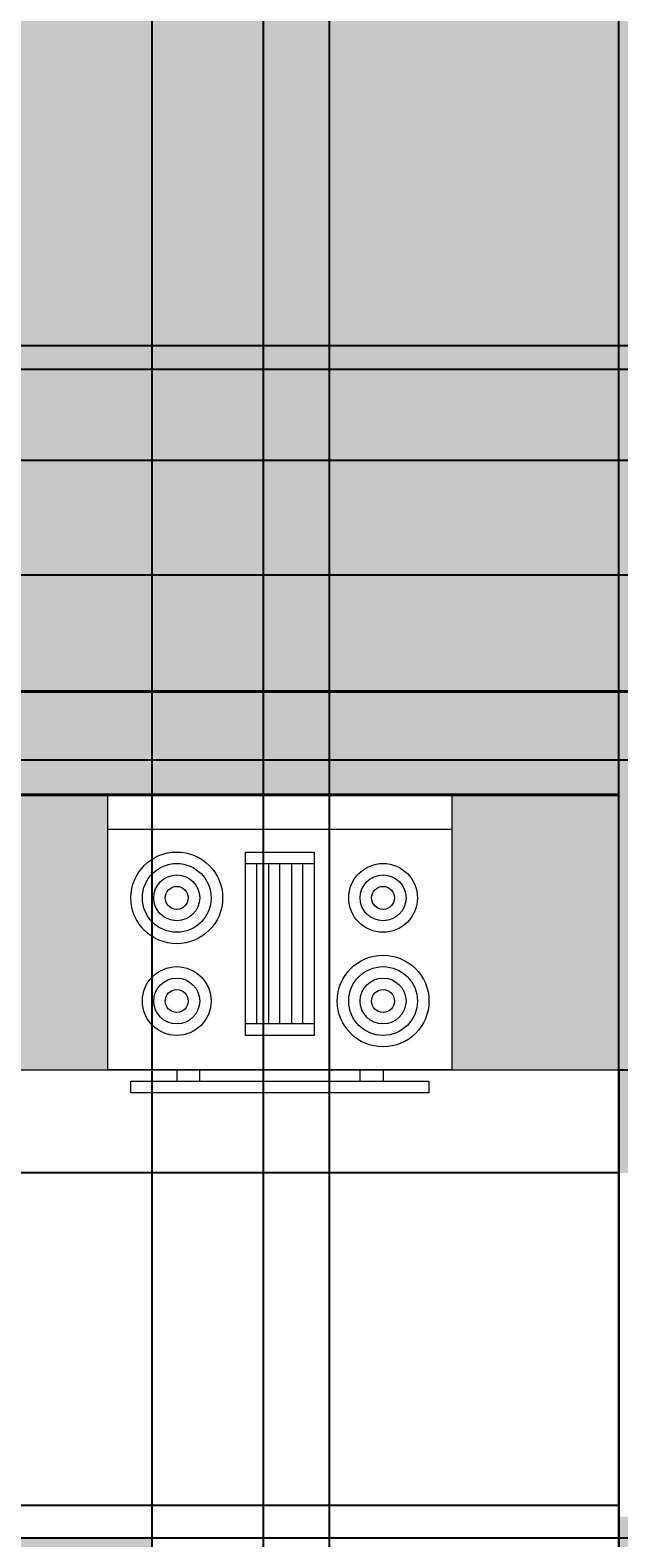
# Model space of a CAD drawing. Units: inches. Extents: x 818 to 1898, y 976 to 2364.
# Tile 87 of 96: x 1539 to 1591, y 1979 to 2111. Entities that reach past the tile are written whole.
import ezdxf

# ---------------------------------------------------------------- set-up
doc = ezdxf.new("R2010")
doc.units = ezdxf.units.IN
doc.header["$LTSCALE"] = 5
doc.header["$MEASUREMENT"] = 0
for name, color, linetype, lineweight in [('A-ANNO-DIMS', 2, 'Continuous', 18), ('A-EQPM', 8, 'Continuous', 18), ('A-FLOR-CASE', 8, 'Continuous', 18), ('A-FURN-PATT', 8, 'Continuous', 9), ('A-WALL', 7, 'Continuous', 40)]:
    doc.layers.add(name, color=color, linetype=linetype, lineweight=lineweight)
doc.layers.add('A-WALL-PATT', color=251, linetype='Continuous', lineweight=13, true_color=0x636466)
doc.layers.add('L-PLNT-PATT', color=114, linetype='Continuous', lineweight=9, true_color=0x139b48)
doc.styles.get("Standard").update_dxf_attribs({"font": 'arial.ttf'})
doc.dimstyles.get("Standard").update_dxf_attribs({"dimtxt": 0.18, "dimasz": 0.18, "dimexe": 0.18, "dimexo": 0.0625, "dimgap": 0.09, "dimtad": 0, "dimtih": 1, "dimtoh": 1, "dimdec": 4, "dimzin": 0, "dimdsep": 46, "dimtxsty": 'Standard', "dimcen": 0.09, "dimadec": 0, "dimazin": 0, "dimtfac": 1, "dimtdec": 4, "dimtofl": 0, "dimtmove": 0, "dimatfit": 3, "dimfxl": 1, "dimtolj": 1, "dimtzin": 0, "dimarcsym": 0})

# ---------------------------------------------------------------- blocks, each defined once
blk = doc.blocks.new('Range-Oven - 30 in top')
for p, q in [((0, -3), (30, -3)), ((12, -6), (18, -6)), ((13, -20), (13, -6)), ((14, -6), (14, -20)), ((15, -20), (15, -6)), ((16, -6), (16, -20)), ((17, -20), (17, -6)), ((18, -20), (12, -20)), ((6, -24), (6, -25)), ((8, -25), (8, -24)), ((22, -25), (22, -24)), ((24, -24), (24, -25))]:
    blk.add_line(p, q)
for points in [[(0, -24), (0, 0), (30, 0), (30, -24)], [(12, -21), (12, -5), (18, -5), (18, -21)], [(2, -26), (2, -25), (28, -25), (28, -26)]]:
    blk.add_lwpolyline(points, close=True)
for centre, radius in [((6, -9), 4), ((6, -9), 3), ((24, -9), 3), ((6, -9), 2), ((24, -9), 2), ((6, -9), 1), ((24, -9), 1), ((24, -18), 4), ((6, -18), 3), ((24, -18), 3), ((6, -18), 2), ((6, -18), 1), ((24, -18), 2), ((24, -18), 1)]:
    blk.add_circle(centre, radius)
blk = doc.blocks.new('*D73')
at = {"layer": 'A-ANNO-DIMS', "color": 0, "lineweight": -2, "ltscale": 5, "transparency": 16777216}
for p, q in [((1590.66, 2011.08), (818.03, 2011.08)), ((818.21, 2010.9), (818.21, 1996.76)), ((818.21, 1982.26), (818.21, 1996.4)), ((1590.66, 1982.08), (818.03, 1982.08))]:
    blk.add_line(p, q, dxfattribs=at)
at = {"layer": 'A-ANNO-DIMS', "color": 0, "ltscale": 5, "transparency": 16777216}
for points in [[(818.18, 2010.9), (818.24, 2010.9), (818.21, 2011.08)], [(818.18, 1982.26), (818.24, 1982.26), (818.21, 1982.08)]]:
    blk.add_solid(points, dxfattribs=at)
at = {"layer": 'Defpoints', "color": 0, "ltscale": 5, "transparency": 16777216}
for p in [(818.21, 2011.08), (1590.73, 2011.08), (1590.73, 1982.08)]:
    blk.add_point(p, dxfattribs=at)
at = {"layer": 'A-ANNO-DIMS', "color": 0, "ltscale": 5, "transparency": 16777216, "insert": (818.21, 1996.58), "char_height": 0.18, "attachment_point": 5}
blk.add_mtext('\\A1;29', dxfattribs=at)
blk = doc.blocks.new('*D85')
at = {"layer": 'A-ANNO-DIMS', "color": 0, "lineweight": -2, "ltscale": 5, "transparency": 16777216}
for p, q in [((1258.79, 2053.08), (1897.92, 2053.08)), ((1897.74, 2052.9), (1897.74, 1876.76)), ((1897.74, 1700.26), (1897.74, 1876.4)), ((1258.79, 1700.08), (1897.92, 1700.08))]:
    blk.add_line(p, q, dxfattribs=at)
at = {"layer": 'A-ANNO-DIMS', "color": 0, "ltscale": 5, "transparency": 16777216}
for points in [[(1897.71, 2052.9), (1897.77, 2052.9), (1897.74, 2053.08)], [(1897.71, 1700.26), (1897.77, 1700.26), (1897.74, 1700.08)]]:
    blk.add_solid(points, dxfattribs=at)
at = {"layer": 'Defpoints', "color": 0, "ltscale": 5, "transparency": 16777216}
for p in [(1258.73, 2053.08), (1897.74, 2053.08), (1258.73, 1700.08)]:
    blk.add_point(p, dxfattribs=at)
at = {"layer": 'A-ANNO-DIMS', "color": 0, "ltscale": 5, "transparency": 16777216, "insert": (1897.74, 1876.58), "char_height": 0.18, "attachment_point": 5}
blk.add_mtext('\\A1;353', dxfattribs=at)
blk = doc.blocks.new('*D86')
at = {"layer": 'A-ANNO-DIMS', "color": 0, "lineweight": -2, "ltscale": 5, "transparency": 16777216}
for p, q in [((1258.73, 2053.14), (1258.73, 2363.87)), ((1714.73, 2053.14), (1714.73, 2363.87)), ((1258.91, 2363.69), (1486.43, 2363.69)), ((1714.55, 2363.69), (1487.02, 2363.69))]:
    blk.add_line(p, q, dxfattribs=at)
at = {"layer": 'A-ANNO-DIMS', "color": 0, "ltscale": 5, "transparency": 16777216}
for points in [[(1258.91, 2363.72), (1258.91, 2363.66), (1258.73, 2363.69)], [(1714.55, 2363.72), (1714.55, 2363.66), (1714.73, 2363.69)]]:
    blk.add_solid(points, dxfattribs=at)
at = {"layer": 'Defpoints', "color": 0, "ltscale": 5, "transparency": 16777216}
for p in [(1714.73, 2363.69), (1258.73, 2053.08), (1714.73, 2053.08)]:
    blk.add_point(p, dxfattribs=at)
at = {"layer": 'A-ANNO-DIMS', "color": 0, "ltscale": 5, "transparency": 16777216, "insert": (1486.73, 2363.69), "char_height": 0.18, "attachment_point": 5}
blk.add_mtext('\\A1;456', dxfattribs=at)
blk = doc.blocks.new('*D101')
at = {"layer": 'A-ANNO-DIMS', "color": 0, "lineweight": -2, "ltscale": 5, "transparency": 16777216}
for p, q in [((1507.3, 1071.12), (1507.3, 2363.87)), ((1565.48, 1071.12), (1565.48, 2363.87)), ((1507.48, 2363.69), (1536, 2363.69)), ((1565.3, 2363.69), (1536.78, 2363.69))]:
    blk.add_line(p, q, dxfattribs=at)
at = {"layer": 'A-ANNO-DIMS', "color": 0, "ltscale": 5, "transparency": 16777216}
for points in [[(1507.48, 2363.72), (1507.48, 2363.66), (1507.3, 2363.69)], [(1565.3, 2363.72), (1565.3, 2363.66), (1565.48, 2363.69)]]:
    blk.add_solid(points, dxfattribs=at)
at = {"layer": 'Defpoints', "color": 0, "ltscale": 5, "transparency": 16777216}
for p in [(1565.48, 2363.69), (1507.3, 1071.06), (1565.48, 1071.06)]:
    blk.add_point(p, dxfattribs=at)
at = {"layer": 'A-ANNO-DIMS', "color": 0, "ltscale": 5, "transparency": 16777216, "insert": (1536.39, 2363.69), "char_height": 0.18, "attachment_point": 5}
blk.add_mtext('\\A1;58.19', dxfattribs=at)
blk = doc.blocks.new('*D102')
at = {"layer": 'A-ANNO-DIMS', "color": 0, "lineweight": -2, "ltscale": 5, "transparency": 16777216}
for p, q in [((1565.48, 1071.12), (1565.48, 2363.87)), ((1626.57, 1071.12), (1626.57, 2363.87)), ((1565.66, 2363.69), (1595.63, 2363.69)), ((1626.39, 2363.69), (1596.42, 2363.69))]:
    blk.add_line(p, q, dxfattribs=at)
at = {"layer": 'A-ANNO-DIMS', "color": 0, "ltscale": 5, "transparency": 16777216}
for points in [[(1565.66, 2363.72), (1565.66, 2363.66), (1565.48, 2363.69)], [(1626.39, 2363.72), (1626.39, 2363.66), (1626.57, 2363.69)]]:
    blk.add_solid(points, dxfattribs=at)
at = {"layer": 'Defpoints', "color": 0, "ltscale": 5, "transparency": 16777216}
for p in [(1626.57, 2363.69), (1565.48, 1071.06), (1626.57, 1071.06)]:
    blk.add_point(p, dxfattribs=at)
at = {"layer": 'A-ANNO-DIMS', "color": 0, "ltscale": 5, "transparency": 16777216, "insert": (1596.03, 2363.69), "char_height": 0.18, "attachment_point": 5}
blk.add_mtext('\\A1;61.09', dxfattribs=at)
blk = doc.blocks.new('*D141')
at = {"layer": 'A-ANNO-DIMS', "color": 0, "lineweight": -2, "ltscale": 5, "transparency": 16777216}
for p, q in [((1218.17, 2083.26), (1897.92, 2083.26)), ((1897.74, 2083.08), (1897.74, 2073.44)), ((1897.74, 2063.44), (1897.74, 2073.08)), ((1198.17, 2063.26), (1897.92, 2063.26))]:
    blk.add_line(p, q, dxfattribs=at)
at = {"layer": 'A-ANNO-DIMS', "color": 0, "ltscale": 5, "transparency": 16777216}
for points in [[(1897.71, 2083.08), (1897.77, 2083.08), (1897.74, 2083.26)], [(1897.71, 2063.44), (1897.77, 2063.44), (1897.74, 2063.26)]]:
    blk.add_solid(points, dxfattribs=at)
at = {"layer": 'Defpoints', "color": 0, "ltscale": 5, "transparency": 16777216}
for p in [(1218.11, 2083.26), (1198.11, 2063.26), (1897.74, 2063.26)]:
    blk.add_point(p, dxfattribs=at)
at = {"layer": 'A-ANNO-DIMS', "color": 0, "ltscale": 5, "transparency": 16777216, "insert": (1897.74, 2073.26), "char_height": 0.18, "attachment_point": 5}
blk.add_mtext('\\A1;20', dxfattribs=at)
blk = doc.blocks.new('*D142')
at = {"layer": 'A-ANNO-DIMS', "color": 0, "lineweight": -2, "ltscale": 5, "transparency": 16777216}
for p, q in [((1208.17, 2073.26), (1897.92, 2073.26)), ((1897.74, 2073.08), (1897.74, 2068.44)), ((1897.74, 2063.44), (1897.74, 2068.08)), ((1198.17, 2063.26), (1897.92, 2063.26))]:
    blk.add_line(p, q, dxfattribs=at)
at = {"layer": 'A-ANNO-DIMS', "color": 0, "ltscale": 5, "transparency": 16777216}
for points in [[(1897.71, 2073.08), (1897.77, 2073.08), (1897.74, 2073.26)], [(1897.71, 2063.44), (1897.77, 2063.44), (1897.74, 2063.26)]]:
    blk.add_solid(points, dxfattribs=at)
at = {"layer": 'Defpoints', "color": 0, "ltscale": 5, "transparency": 16777216}
for p in [(1208.11, 2073.26), (1897.74, 2073.26), (1198.11, 2063.26)]:
    blk.add_point(p, dxfattribs=at)
at = {"layer": 'A-ANNO-DIMS', "color": 0, "ltscale": 5, "transparency": 16777216, "insert": (1897.74, 2068.26), "char_height": 0.18, "attachment_point": 5}
blk.add_mtext('\\A1;10', dxfattribs=at)
blk = doc.blocks.new('*D161')
at = {"layer": 'A-ANNO-DIMS', "color": 0, "lineweight": -2, "ltscale": 5, "transparency": 16777216}
for p, q in [((1429.23, 1876.14), (1429.23, 2363.87)), ((1590.73, 1876.14), (1590.73, 2363.87)), ((1429.41, 2363.69), (1509.59, 2363.69)), ((1590.55, 2363.69), (1510.36, 2363.69))]:
    blk.add_line(p, q, dxfattribs=at)
at = {"layer": 'A-ANNO-DIMS', "color": 0, "ltscale": 5, "transparency": 16777216}
for points in [[(1429.41, 2363.72), (1429.41, 2363.66), (1429.23, 2363.69)], [(1590.55, 2363.72), (1590.55, 2363.66), (1590.73, 2363.69)]]:
    blk.add_solid(points, dxfattribs=at)
at = {"layer": 'Defpoints', "color": 0, "ltscale": 5, "transparency": 16777216}
for p in [(1590.73, 2363.69), (1429.23, 1876.08), (1590.73, 1876.08)]:
    blk.add_point(p, dxfattribs=at)
at = {"layer": 'A-ANNO-DIMS', "color": 0, "ltscale": 5, "transparency": 16777216, "insert": (1509.98, 2363.69), "char_height": 0.18, "attachment_point": 5}
blk.add_mtext('\\A1;161.5', dxfattribs=at)
blk = doc.blocks.new('*D175')
at = {"layer": 'A-ANNO-DIMS', "color": 0, "lineweight": -2, "ltscale": 5, "transparency": 16777216}
for p, q in [((1559.73, 1647.64), (1559.73, 2363.87)), ((1669.73, 1647.64), (1669.73, 2363.87)), ((1559.91, 2363.69), (1614.45, 2363.69)), ((1669.55, 2363.69), (1615.01, 2363.69))]:
    blk.add_line(p, q, dxfattribs=at)
at = {"layer": 'A-ANNO-DIMS', "color": 0, "ltscale": 5, "transparency": 16777216}
for points in [[(1559.91, 2363.72), (1559.91, 2363.66), (1559.73, 2363.69)], [(1669.55, 2363.72), (1669.55, 2363.66), (1669.73, 2363.69)]]:
    blk.add_solid(points, dxfattribs=at)
at = {"layer": 'Defpoints', "color": 0, "ltscale": 5, "transparency": 16777216}
for p in [(1669.73, 2363.69), (1559.73, 1647.58), (1669.73, 1647.58)]:
    blk.add_point(p, dxfattribs=at)
at = {"layer": 'A-ANNO-DIMS', "color": 0, "ltscale": 5, "transparency": 16777216, "insert": (1614.73, 2363.69), "char_height": 0.18, "attachment_point": 5}
blk.add_mtext('\\A1;110', dxfattribs=at)
blk = doc.blocks.new('*D205')
at = {"layer": 'A-ANNO-DIMS', "color": 0, "lineweight": -2, "ltscale": 5, "transparency": 16777216}
for p, q in [((1590.73, 2044.14), (1590.73, 2363.87)), ((1714.73, 2053.14), (1714.73, 2363.87)), ((1590.91, 2363.69), (1652.45, 2363.69)), ((1714.55, 2363.69), (1653.01, 2363.69))]:
    blk.add_line(p, q, dxfattribs=at)
at = {"layer": 'A-ANNO-DIMS', "color": 0, "ltscale": 5, "transparency": 16777216}
for points in [[(1590.91, 2363.72), (1590.91, 2363.66), (1590.73, 2363.69)], [(1714.55, 2363.72), (1714.55, 2363.66), (1714.73, 2363.69)]]:
    blk.add_solid(points, dxfattribs=at)
at = {"layer": 'Defpoints', "color": 0, "ltscale": 5, "transparency": 16777216}
for p in [(1714.73, 2363.69), (1714.73, 2053.08), (1590.73, 2044.08)]:
    blk.add_point(p, dxfattribs=at)
at = {"layer": 'A-ANNO-DIMS', "color": 0, "ltscale": 5, "transparency": 16777216, "insert": (1652.73, 2363.69), "char_height": 0.18, "attachment_point": 5}
blk.add_mtext('\\A1;124', dxfattribs=at)
blk = doc.blocks.new('*D207')
at = {"layer": 'A-ANNO-DIMS', "color": 0, "lineweight": -2, "ltscale": 5, "transparency": 16777216}
for p, q in [((1590.66, 2044.08), (818.03, 2044.08)), ((818.21, 2043.9), (818.21, 2027.76)), ((818.21, 2011.26), (818.21, 2027.4)), ((1590.66, 2011.08), (818.03, 2011.08))]:
    blk.add_line(p, q, dxfattribs=at)
at = {"layer": 'A-ANNO-DIMS', "color": 0, "ltscale": 5, "transparency": 16777216}
for points in [[(818.18, 2043.9), (818.24, 2043.9), (818.21, 2044.08)], [(818.18, 2011.26), (818.24, 2011.26), (818.21, 2011.08)]]:
    blk.add_solid(points, dxfattribs=at)
at = {"layer": 'Defpoints', "color": 0, "ltscale": 5, "transparency": 16777216}
for p in [(818.21, 2044.08), (1590.73, 2044.08), (1590.73, 2011.08)]:
    blk.add_point(p, dxfattribs=at)
at = {"layer": 'A-ANNO-DIMS', "color": 0, "ltscale": 5, "transparency": 16777216, "insert": (818.21, 2027.58), "char_height": 0.18, "attachment_point": 5}
blk.add_mtext('\\A1;33', dxfattribs=at)
blk = doc.blocks.new('*D238')
at = {"layer": 'A-ANNO-DIMS', "color": 0, "lineweight": -2, "ltscale": 5, "transparency": 16777216}
for p, q in [((1483.55, 1948.72), (1483.55, 2363.87)), ((1550.01, 1948.72), (1550.01, 2363.87)), ((1483.73, 2363.69), (1516.38, 2363.69)), ((1549.83, 2363.69), (1517.17, 2363.69))]:
    blk.add_line(p, q, dxfattribs=at)
at = {"layer": 'A-ANNO-DIMS', "color": 0, "ltscale": 5, "transparency": 16777216}
for points in [[(1483.73, 2363.72), (1483.73, 2363.66), (1483.55, 2363.69)], [(1549.83, 2363.72), (1549.83, 2363.66), (1550.01, 2363.69)]]:
    blk.add_solid(points, dxfattribs=at)
at = {"layer": 'Defpoints', "color": 0, "ltscale": 5, "transparency": 16777216}
for p in [(1550.01, 2363.69), (1483.55, 1948.66), (1550.01, 1948.66)]:
    blk.add_point(p, dxfattribs=at)
at = {"layer": 'A-ANNO-DIMS', "color": 0, "ltscale": 5, "transparency": 16777216, "insert": (1516.78, 2363.69), "char_height": 0.18, "attachment_point": 5}
blk.add_mtext('\\A1;66.47', dxfattribs=at)
blk = doc.blocks.new('*D239')
at = {"layer": 'A-ANNO-DIMS', "color": 0, "lineweight": -2, "ltscale": 5, "transparency": 16777216}
for p, q in [((1483.61, 1979.24), (1897.92, 1979.24)), ((1897.74, 1979.06), (1897.74, 1964.13)), ((1897.74, 1948.84), (1897.74, 1963.77)), ((1483.61, 1948.66), (1897.92, 1948.66))]:
    blk.add_line(p, q, dxfattribs=at)
at = {"layer": 'A-ANNO-DIMS', "color": 0, "ltscale": 5, "transparency": 16777216}
for points in [[(1897.71, 1979.06), (1897.77, 1979.06), (1897.74, 1979.24)], [(1897.71, 1948.84), (1897.77, 1948.84), (1897.74, 1948.66)]]:
    blk.add_solid(points, dxfattribs=at)
at = {"layer": 'Defpoints', "color": 0, "ltscale": 5, "transparency": 16777216}
for p in [(1483.55, 1979.24), (1897.74, 1979.24), (1483.55, 1948.66)]:
    blk.add_point(p, dxfattribs=at)
at = {"layer": 'A-ANNO-DIMS', "color": 0, "ltscale": 5, "transparency": 16777216, "insert": (1897.74, 1963.95), "char_height": 0.18, "attachment_point": 5}
blk.add_mtext('\\A1;30.584', dxfattribs=at)
blk = doc.blocks.new('*D240')
at = {"layer": 'A-ANNO-DIMS', "color": 0, "lineweight": -2, "ltscale": 5, "transparency": 16777216}
for p, q in [((1550.01, 1979.31), (1550.01, 2363.87)), ((1590.73, 1981.14), (1590.73, 2363.87)), ((1550.19, 2363.69), (1569.9, 2363.69)), ((1590.55, 2363.69), (1570.83, 2363.69))]:
    blk.add_line(p, q, dxfattribs=at)
at = {"layer": 'A-ANNO-DIMS', "color": 0, "ltscale": 5, "transparency": 16777216}
for points in [[(1550.19, 2363.72), (1550.19, 2363.66), (1550.01, 2363.69)], [(1590.55, 2363.72), (1590.55, 2363.66), (1590.73, 2363.69)]]:
    blk.add_solid(points, dxfattribs=at)
at = {"layer": 'Defpoints', "color": 0, "ltscale": 5, "transparency": 16777216}
for p in [(1590.73, 2363.69), (1590.73, 1981.08), (1550.01, 1979.24)]:
    blk.add_point(p, dxfattribs=at)
at = {"layer": 'A-ANNO-DIMS', "color": 0, "ltscale": 5, "transparency": 16777216, "insert": (1570.37, 2363.69), "char_height": 0.18, "attachment_point": 5}
blk.add_mtext('\\A1;40.714', dxfattribs=at)
blk = doc.blocks.new('*D241')
at = {"layer": 'A-ANNO-DIMS', "color": 0, "lineweight": -2, "ltscale": 5, "transparency": 16777216}
for p, q in [((1590.79, 2020.08), (1897.92, 2020.08)), ((1897.74, 2019.9), (1897.74, 1999.84)), ((1897.74, 1979.42), (1897.74, 1999.48)), ((1550.07, 1979.24), (1897.92, 1979.24))]:
    blk.add_line(p, q, dxfattribs=at)
at = {"layer": 'A-ANNO-DIMS', "color": 0, "ltscale": 5, "transparency": 16777216}
for points in [[(1897.71, 2019.9), (1897.77, 2019.9), (1897.74, 2020.08)], [(1897.71, 1979.42), (1897.77, 1979.42), (1897.74, 1979.24)]]:
    blk.add_solid(points, dxfattribs=at)
at = {"layer": 'Defpoints', "color": 0, "ltscale": 5, "transparency": 16777216}
for p in [(1590.73, 2020.08), (1897.74, 2020.08), (1550.01, 1979.24)]:
    blk.add_point(p, dxfattribs=at)
at = {"layer": 'A-ANNO-DIMS', "color": 0, "ltscale": 5, "transparency": 16777216, "insert": (1897.74, 1999.66), "char_height": 0.18, "attachment_point": 5}
blk.add_mtext('\\A1;40.83', dxfattribs=at)
blk = doc.blocks.new('*D243')
at = {"layer": 'A-ANNO-DIMS', "color": 0, "lineweight": -2, "ltscale": 5, "transparency": 16777216}
for p, q in [((1451.77, 2020.02), (1451.77, 975.66)), ((1590.73, 2020.02), (1590.73, 975.66)), ((1451.95, 975.84), (1520.79, 975.84)), ((1590.55, 975.84), (1521.7, 975.84))]:
    blk.add_line(p, q, dxfattribs=at)
at = {"layer": 'A-ANNO-DIMS', "color": 0, "ltscale": 5, "transparency": 16777216}
for points in [[(1451.95, 975.87), (1451.95, 975.81), (1451.77, 975.84)], [(1590.55, 975.87), (1590.55, 975.81), (1590.73, 975.84)]]:
    blk.add_solid(points, dxfattribs=at)
at = {"layer": 'Defpoints', "color": 0, "ltscale": 5, "transparency": 16777216}
for p in [(1451.77, 2020.08), (1590.73, 2020.08), (1590.73, 975.84)]:
    blk.add_point(p, dxfattribs=at)
at = {"layer": 'A-ANNO-DIMS', "color": 0, "ltscale": 5, "transparency": 16777216, "insert": (1521.25, 975.84), "char_height": 0.18, "attachment_point": 5}
blk.add_mtext('\\A1;138.96', dxfattribs=at)
blk = doc.blocks.new('*D244')
at = {"layer": 'A-ANNO-DIMS', "color": 0, "lineweight": -2, "ltscale": 5, "transparency": 16777216}
for p, q in [((1519.64, 1900.14), (1519.64, 2363.87)), ((1590.73, 1900.14), (1590.73, 2363.87)), ((1519.82, 2363.69), (1554.79, 2363.69)), ((1590.55, 2363.69), (1555.58, 2363.69))]:
    blk.add_line(p, q, dxfattribs=at)
at = {"layer": 'A-ANNO-DIMS', "color": 0, "ltscale": 5, "transparency": 16777216}
for points in [[(1519.82, 2363.72), (1519.82, 2363.66), (1519.64, 2363.69)], [(1590.55, 2363.72), (1590.55, 2363.66), (1590.73, 2363.69)]]:
    blk.add_solid(points, dxfattribs=at)
at = {"layer": 'Defpoints', "color": 0, "ltscale": 5, "transparency": 16777216}
for p in [(1590.73, 2363.69), (1519.64, 1900.08), (1590.73, 1900.08)]:
    blk.add_point(p, dxfattribs=at)
at = {"layer": 'A-ANNO-DIMS', "color": 0, "ltscale": 5, "transparency": 16777216, "insert": (1555.18, 2363.69), "char_height": 0.18, "attachment_point": 5}
blk.add_mtext('\\A1;71.08', dxfattribs=at)
blk = doc.blocks.new('*D266')
at = {"layer": 'A-ANNO-DIMS', "color": 0, "lineweight": -2, "ltscale": 5, "transparency": 16777216}
for p, q in [((1780.44, 2053.08), (818.03, 2053.08)), ((818.21, 2052.9), (818.21, 2050.26)), ((818.21, 2047.26), (818.21, 2049.9)), ((1780.44, 2047.08), (818.03, 2047.08))]:
    blk.add_line(p, q, dxfattribs=at)
at = {"layer": 'A-ANNO-DIMS', "color": 0, "ltscale": 5, "transparency": 16777216}
for points in [[(818.18, 2052.9), (818.24, 2052.9), (818.21, 2053.08)], [(818.18, 2047.26), (818.24, 2047.26), (818.21, 2047.08)]]:
    blk.add_solid(points, dxfattribs=at)
at = {"layer": 'Defpoints', "color": 0, "ltscale": 5, "transparency": 16777216}
for p in [(1780.5, 2053.08), (818.21, 2047.08), (1780.5, 2047.08)]:
    blk.add_point(p, dxfattribs=at)
at = {"layer": 'A-ANNO-DIMS', "color": 0, "ltscale": 5, "transparency": 16777216, "insert": (818.21, 2050.08), "char_height": 0.18, "attachment_point": 5}
blk.add_mtext('\\A1;6', dxfattribs=at)
blk = doc.blocks.new('*D281')
at = {"layer": 'A-ANNO-DIMS', "color": 0, "lineweight": -2, "ltscale": 5, "transparency": 16777216}
for p, q in [((1250.3, 1913.7), (1250.3, 2363.87)), ((1590.73, 2011.14), (1590.73, 2363.87)), ((1250.48, 2363.69), (1420.12, 2363.69)), ((1590.55, 2363.69), (1420.91, 2363.69))]:
    blk.add_line(p, q, dxfattribs=at)
at = {"layer": 'A-ANNO-DIMS', "color": 0, "ltscale": 5, "transparency": 16777216}
for points in [[(1250.48, 2363.72), (1250.48, 2363.66), (1250.3, 2363.69)], [(1590.55, 2363.72), (1590.55, 2363.66), (1590.73, 2363.69)]]:
    blk.add_solid(points, dxfattribs=at)
at = {"layer": 'Defpoints', "color": 0, "ltscale": 5, "transparency": 16777216}
for p in [(1590.73, 2363.69), (1590.73, 2011.08), (1250.3, 1913.64)]:
    blk.add_point(p, dxfattribs=at)
at = {"layer": 'A-ANNO-DIMS', "color": 0, "ltscale": 5, "transparency": 16777216, "insert": (1420.51, 2363.69), "char_height": 0.18, "attachment_point": 5}
blk.add_mtext('\\A1;340.4', dxfattribs=at)
blk = doc.blocks.new('*D282')
at = {"layer": 'A-ANNO-DIMS', "color": 0, "lineweight": -2, "ltscale": 5, "transparency": 16777216}
for p, q in [((1422.08, 2081.19), (1897.92, 2081.19)), ((1897.74, 2081.01), (1897.74, 1884.32)), ((1897.74, 1687.26), (1897.74, 1883.95)), ((1463.79, 1687.08), (1897.92, 1687.08))]:
    blk.add_line(p, q, dxfattribs=at)
at = {"layer": 'A-ANNO-DIMS', "color": 0, "ltscale": 5, "transparency": 16777216}
for points in [[(1897.71, 2081.01), (1897.77, 2081.01), (1897.74, 2081.19)], [(1897.71, 1687.26), (1897.77, 1687.26), (1897.74, 1687.08)]]:
    blk.add_solid(points, dxfattribs=at)
at = {"layer": 'Defpoints', "color": 0, "ltscale": 5, "transparency": 16777216}
for p in [(1422.02, 2081.19), (1897.74, 2081.19), (1463.73, 1687.08)]:
    blk.add_point(p, dxfattribs=at)
at = {"layer": 'A-ANNO-DIMS', "color": 0, "ltscale": 5, "transparency": 16777216, "insert": (1897.74, 1884.13), "char_height": 0.18, "attachment_point": 5}
blk.add_mtext('\\A1;394.1', dxfattribs=at)

msp = doc.modelspace()

# ---------------------------------------------------------------- hatches: boundary and pattern name
at = {"layer": 'A-FURN-PATT', "ltscale": 5}
h = msp.add_hatch(color=256, dxfattribs=at)
h.dxf.hatch_style = 1
h.paths.add_polyline_path([(1341.9997, 1981.5338), (1317.9034, 2001.8247), (1314.2595, 2001.8247), (1314.2595, 2004.893), (1310.1046, 2008.3917), (1303.9314, 2008.3917), (1303.9314, 1953.0408), (1308.1629, 1953.0408), (1314.2595, 1958.1746), (1314.2595, 1959.6079), (1315.9616, 1959.6079)])
h.paths.add_polyline_path([(1341.9997, 1981.5338), (1315.9616, 1959.6079), (1336.7936, 1959.6079), (1336.7936, 1953.0408), (1345.3966, 1953.0408), (1345.3966, 1959.6079), (1368.0379, 1959.6079)])
h.paths.add_polyline_path([(1402.518, 2008.3917), (1398.8475, 2008.3917), (1398.8475, 2001.8247), (1376.3134, 2001.8247), (1376.3134, 2008.3917), (1373.8948, 2008.3917), (1367.9307, 2003.3695), (1367.9307, 2001.8247), (1366.0961, 2001.8247), (1341.9997, 1981.5338), (1368.0379, 1959.6079), (1375.8366, 1953.0408), (1376.3134, 1953.0408), (1376.3134, 1959.6079), (1398.8475, 1959.6079), (1398.8475, 1953.0408), (1402.518, 1953.0408)])
h.paths.add_polyline_path([(1366.0961, 2001.8247), (1345.3966, 2001.8247), (1345.3966, 2008.3917), (1336.7936, 2008.3917), (1336.7936, 2001.8247), (1317.9034, 2001.8247), (1341.9997, 1981.5338)])
h.paths.add_polyline_path([(1336.7936, 1959.6079), (1315.9616, 1959.6079), (1314.2595, 1958.1746), (1314.2595, 1953.0408), (1336.7936, 1953.0408)], flags=17)
h.paths.add_polyline_path([(1367.9307, 1959.6079), (1345.3966, 1959.6079), (1345.3966, 1953.0408), (1367.9307, 1953.0408)], flags=17)
h.paths.add_polyline_path([(1398.8475, 1959.6079), (1376.3134, 1959.6079), (1376.3134, 1953.0408), (1398.8475, 1953.0408)], flags=17)
h.paths.add_polyline_path([(1368.0379, 1959.6079), (1367.9307, 1959.6079), (1367.9307, 1953.0408), (1375.8366, 1953.0408)], flags=17)
h.paths.add_polyline_path([(1314.2595, 1958.1746), (1308.1629, 1953.0408), (1314.2595, 1953.0408)], flags=17)
h.paths.add_polyline_path([(1315.9616, 1959.6079), (1314.2595, 1959.6079), (1314.2595, 1958.1746)], flags=16)
h.paths.add_polyline_path([(1314.2595, 2008.3917), (1310.1046, 2008.3917), (1314.2595, 2004.893)], flags=17)
h.paths.add_polyline_path([(1336.7936, 2008.3917), (1314.2595, 2008.3917), (1314.2595, 2004.893), (1317.9034, 2001.8247), (1336.7936, 2001.8247)], flags=17)
h.paths.add_polyline_path([(1314.2595, 2004.893), (1314.2595, 2001.8247), (1317.9034, 2001.8247)], flags=16)
h.paths.add_polyline_path([(1367.9307, 2008.3917), (1345.3966, 2008.3917), (1345.3966, 2001.8247), (1366.0961, 2001.8247), (1367.9307, 2003.3695)], flags=17)
h.paths.add_polyline_path([(1398.8475, 2008.3917), (1376.3134, 2008.3917), (1376.3134, 2001.8247), (1398.8475, 2001.8247)], flags=17)
h.paths.add_polyline_path([(1373.8948, 2008.3917), (1367.9307, 2008.3917), (1367.9307, 2003.3695)], flags=17)
h.paths.add_polyline_path([(1367.9307, 2003.3695), (1366.0961, 2001.8247), (1367.9307, 2001.8247)], flags=16)
h.paths.add_polyline_path([(1546.1595, 2044.0782), (1451.7698, 2044.0782), (1451.7698, 2020.0782), (1546.1595, 2020.0782)])
h.paths.add_polyline_path([(1492.0729, 2040.001, 0.431429), (1491.8238, 2040.251), (1491.3087, 2040.251, 0.41521699), (1491.0729, 2040.001)], flags=16)
h.paths.add_polyline_path([(1481.8346, 2039.6036), (1511.886, 2039.6036), (1511.886, 2024.9917), (1481.8346, 2024.9917)], flags=16)
h.paths.add_polyline_path([(1491.0729, 2039.4857), (1491.0729, 2039.501), (1492.0729, 2039.501, -0.41174844), (1491.8401, 2039.251), (1491.8229, 2039.251), (1491.8229, 2039.2509, 0.43259178), (1492.0729, 2039.501), (1491.0729, 2039.501, 0.43260402), (1491.3229, 2039.2509), (1491.3229, 2039.251), (1491.325, 2039.251, -0.41658228)], flags=0)
h.paths.add_polyline_path([(1485.3701, 2030.9622), (1485.3701, 2034.3556, -0.41421356), (1488.3701, 2037.3556), (1490.3421, 2037.3556, -0.07791932), (1491.0729, 2038.751), (1495.0729, 2038.751, -0.31486788), (1496.07, 2037.1201, -0.30166092), (1497.9049, 2034.3556), (1497.9049, 2030.9622, -0.41421356), (1494.9049, 2027.9622), (1488.3701, 2027.9622, -0.41421356)], flags=0)
h.paths.add_polyline_path([(1490.3229, 2035.751, 0.26556482), (1491.3229, 2036.751), (1491.3229, 2037.126), (1491.0729, 2037.126, -0.79141832), (1490.5434, 2037.251, -0.79141832), (1491.0729, 2037.376), (1491.3229, 2037.376), (1491.3229, 2037.751), (1492.0729, 2037.751), (1492.0729, 2037.376), (1492.3229, 2037.376, -0.79141832), (1492.8524, 2037.251, -0.79141832), (1492.3229, 2037.126), (1492.1491, 2037.126, -0.08662632), (1492.5376, 2036.0294, 0.10704809), (1493.0729, 2035.751), (1490.3229, 2035.751)], flags=0)
h.paths.add_polyline_path([(1491.9774, 2037.251, -1), (1491.4184, 2037.251, -1)], flags=0)
h.paths.add_polyline_path([(1500.0743, 2028.6045), (1500.0743, 2029.4074), (1510.8414, 2029.4074), (1510.8414, 2028.6045)], flags=0)
h.paths.add_polyline_path([(1500.0743, 2030.5314), (1500.0743, 2031.3342), (1510.8414, 2031.3342), (1510.8414, 2030.5314)], flags=0)
h.paths.add_polyline_path([(1500.0743, 2032.94), (1500.0743, 2033.7428), (1510.8414, 2033.7428), (1510.8414, 2032.94)], flags=0)
h.paths.add_polyline_path([(1500.0743, 2035.7499), (1500.0743, 2036.5528), (1510.8414, 2036.5528), (1510.8414, 2035.7499)], flags=0)
h.paths.add_polyline_path([(1590.7251, 2044.0782), (1576.1595, 2044.0782), (1576.1595, 2020.0782), (1590.7251, 2020.0782)])
h.paths.add_polyline_path([(1668.4429, 2044.0782), (1599.7252, 2044.0782), (1599.7252, 2020.0782), (1668.4429, 2020.0782)])
h.paths.add_polyline_path([(1621.2588, 2040.001, 0.431429), (1621.0097, 2040.251), (1620.4946, 2040.251, 0.41521699), (1620.2588, 2040.001)], flags=16)
h.paths.add_polyline_path([(1611.0205, 2024.9917), (1611.0205, 2039.6036), (1641.0719, 2039.6036), (1641.0719, 2024.9917)], flags=16)
h.paths.add_polyline_path([(1620.2588, 2039.4857), (1620.2588, 2039.501), (1621.2588, 2039.501, -0.41174844), (1621.026, 2039.251), (1621.0088, 2039.251), (1621.0088, 2039.2509, 0.43259178), (1621.2588, 2039.501), (1620.2588, 2039.501, 0.43260402), (1620.5088, 2039.2509), (1620.5088, 2039.251), (1620.5109, 2039.251, -0.41658228)], flags=0)
h.paths.add_polyline_path([(1614.556, 2030.9622), (1614.556, 2034.3556, -0.41421356), (1617.556, 2037.3556), (1619.528, 2037.3556, -0.07791932), (1620.2588, 2038.751), (1624.2588, 2038.751, -0.31486788), (1625.2559, 2037.1201, -0.30166092), (1627.0908, 2034.3556), (1627.0908, 2030.9622, -0.41421356), (1624.0908, 2027.9622), (1617.556, 2027.9622, -0.41421356)], flags=0)
h.paths.add_polyline_path([(1619.5088, 2035.751, 0.26556482), (1620.5088, 2036.751), (1620.5088, 2037.126), (1620.2588, 2037.126, -0.79141832), (1619.7293, 2037.251, -0.79141832), (1620.2588, 2037.376), (1620.5088, 2037.376), (1620.5088, 2037.751), (1621.2588, 2037.751), (1621.2588, 2037.376), (1621.5088, 2037.376, -0.79141832), (1622.0383, 2037.251, -0.79141832), (1621.5088, 2037.126), (1621.335, 2037.126, -0.08662632), (1621.7235, 2036.0294, 0.10704809), (1622.2588, 2035.751), (1619.5088, 2035.751)], flags=0)
h.paths.add_polyline_path([(1620.6043, 2037.251, -1), (1621.1633, 2037.251, -1)], flags=0)
h.paths.add_polyline_path([(1629.2602, 2028.6045), (1629.2602, 2029.4074), (1640.0273, 2029.4074), (1640.0273, 2028.6045)], flags=0)
h.paths.add_polyline_path([(1629.2602, 2030.5314), (1629.2602, 2031.3342), (1640.0273, 2031.3342), (1640.0273, 2030.5314)], flags=0)
h.paths.add_polyline_path([(1629.2602, 2032.94), (1629.2602, 2033.7428), (1640.0273, 2033.7428), (1640.0273, 2032.94)], flags=0)
h.paths.add_polyline_path([(1629.2602, 2035.7499), (1629.2602, 2036.5528), (1640.0273, 2036.5528), (1640.0273, 2035.7499)], flags=0)
h.paths.add_polyline_path([(1705.7252, 2044.0782), (1698.4429, 2044.0782), (1698.4429, 2020.0782), (1705.7252, 2020.0782)])
h.paths.add_polyline_path([(1705.7252, 1972.0782), (1599.7252, 1972.0782), (1599.7252, 1948.0782), (1705.7252, 1948.0782)])
h.paths.add_polyline_path([(1550.0109, 1979.2444), (1483.5451, 1979.2444), (1483.5451, 1948.6602), (1550.0109, 1948.6602)])
h.paths.add_polyline_path([(1490.2586, 1948.6602), (1488.2586, 1948.6602), (1488.2586, 1941.1742, 0.41421356), (1491.2586, 1938.1742), (1500.7446, 1938.1742, -0.41421356)])
h.paths.add_polyline_path([(1513.2306, 1941.1742), (1513.2306, 1948.6602), (1511.2306, 1948.6602, -0.41421356), (1500.7446, 1938.1742), (1510.2306, 1938.1742, 0.41421356)])
h.paths.add_polyline_path([(1518.778, 1948.6602), (1516.778, 1948.6602), (1516.778, 1941.1742, 0.41421356), (1519.778, 1938.1742), (1529.264, 1938.1742, -0.41421356)])
h.paths.add_polyline_path([(1541.75, 1941.1742), (1541.75, 1948.6602), (1539.75, 1948.6602, -0.41421356), (1529.264, 1938.1742), (1538.75, 1938.1742, 0.41421356)])
h.paths.add_polyline_path([(1590.7251, 1900.0782), (1519.6413, 1900.0782), (1519.6413, 1876.0782), (1590.7251, 1876.0782)])
at = {"layer": 'A-WALL-PATT', "ltscale": 5}
h = msp.add_hatch(color=256, dxfattribs=at)
h.dxf.hatch_style = 1
h.paths.add_polyline_path([(1267.7252, 1928.9218), (1258.7251, 1928.9218), (1258.7251, 1913.6401), (1250.3029, 1913.6401), (1250.3029, 1878.3919), (1258.7251, 1878.3919), (1258.7251, 1862.9652), (1267.7252, 1862.9652)])
h.paths.add_polyline_path([(1267.7252, 1814.9652), (1258.7251, 1814.9652), (1258.7251, 1755.3321), (1267.7252, 1755.3321)])
h.paths.add_polyline_path([(1463.7251, 1696.0782), (1267.7252, 1696.0782), (1267.7252, 1707.3321), (1258.7251, 1707.3321), (1258.7251, 1700.0782), (1251.9333, 1700.0782), (1251.9333, 1687.0782), (1463.7251, 1687.0782)])
h.paths.add_polyline_path([(1714.7251, 1717.3178), (1705.7252, 1717.3178), (1705.7252, 1696.0782), (1599.7252, 1696.0782), (1599.7252, 1790.0782), (1705.7252, 1790.0782), (1705.7252, 1785.6125), (1714.7251, 1785.6125), (1714.7251, 1827.2125), (1705.7252, 1827.2125), (1705.7252, 1802.0782), (1599.7252, 1802.0782), (1599.7252, 1867.0782), (1705.7252, 1867.0782), (1705.7252, 1857.2125), (1714.7251, 1857.2125), (1714.7251, 1930.0316), (1741.8409, 1930.0316), (1741.8409, 1935.0316), (1714.7251, 1935.0316), (1714.7251, 1957.0338), (1741.8409, 1957.0338), (1741.8409, 1962.0338), (1714.7251, 1962.0338), (1705.7252, 1962.0338), (1705.7252, 1948.0782), (1599.7252, 1948.0782), (1599.7252, 1981.0782), (1590.7251, 1981.0782), (1590.7251, 1941.0782), (1620.7252, 1941.0782), (1705.7252, 1941.0782), (1705.7252, 1876.0782), (1599.7252, 1876.0782), (1599.7252, 1911.0782), (1590.7251, 1911.0782), (1590.7251, 1876.0782), (1429.2251, 1876.0782), (1429.2251, 1867.0782), (1511.7252, 1867.0782), (1528.593, 1867.0782), (1595.7252, 1867.0782), (1595.7252, 1773.0782), (1520.7252, 1773.0782), (1520.7252, 1837.5823), (1532.593, 1837.5823), (1532.593, 1867.0782), (1528.593, 1867.0782), (1528.593, 1841.5823), (1511.7252, 1841.5823), (1511.7252, 1744.9714), (1520.7252, 1744.9714), (1520.7252, 1761.0782), (1595.7252, 1761.0782), (1595.7252, 1696.0782), (1520.7252, 1696.0782), (1520.7252, 1716.0454), (1511.7252, 1716.0454), (1511.7252, 1696.0782), (1511.7252, 1687.0782), (1714.7251, 1687.0782)])
h.paths.add_polyline_path([(1714.7251, 2053.0782), (1714.7251, 2081.1881), (1709.7252, 2081.1881), (1709.7252, 2053.0782), (1681.6446, 2053.0782), (1681.6446, 2081.1881), (1676.6446, 2081.1881), (1676.6446, 2053.0782), (1538.5155, 2053.0782), (1538.5155, 2044.0782), (1590.7251, 2044.0782), (1590.7251, 2011.0782), (1599.7252, 2011.0782), (1599.7252, 2044.0782), (1705.7252, 2044.0782), (1705.7252, 2014.5114), (1714.7251, 2014.5114)])
h.paths.add_polyline_path([(1485.1216, 2053.0782), (1422.02, 2053.0782), (1422.02, 2081.1881), (1413.02, 2081.1881), (1413.02, 2053.0782), (1399.6356, 2053.0782), (1399.6356, 2081.1881), (1390.6356, 2081.1881), (1390.6356, 2053.0782), (1388.0315, 2053.0782), (1388.0315, 2044.0782), (1416.2743, 2044.0782), (1485.1216, 2044.0782)])
h.paths.add_polyline_path([(1330.305, 2053.0782), (1258.7251, 2053.0782), (1258.7251, 2019.2871), (1267.7252, 2019.2871), (1267.7252, 2044.0782), (1330.305, 2044.0782)])
h.paths.add_polyline_path([(1258.7251, 2053.0782), (1214.6577, 2053.0782), (1214.6577, 2044.0782), (1258.7251, 2044.0782)])
h.paths.add_polyline_path([(1214.6577, 2053.0782), (1180.349, 2053.0782), (1180.349, 2044.0782), (1214.6577, 2044.0782)])
h.paths.add_polyline_path([(1714.7251, 1639.5782), (1741.8409, 1639.5782), (1741.8409, 1643.5782), (1714.7251, 1643.5782), (1714.7251, 1649.9029), (1705.7252, 1649.9029), (1705.7252, 1600.0782), (1477.7252, 1600.0782), (1477.7252, 1591.0782), (1520.7252, 1591.0782), (1616.7252, 1591.0782), (1616.7252, 1416.6857), (1622.7252, 1416.6857), (1622.7252, 1463.0782), (1624.7252, 1463.0782), (1624.7252, 1467.0782), (1622.7252, 1467.0782), (1622.7252, 1591.0782), (1705.7252, 1591.0782), (1705.7252, 1545.0782), (1714.7251, 1545.0782), (1741.8409, 1545.0782), (1741.8409, 1549.0782), (1714.7251, 1549.0782), (1714.7251, 1593.9175), (1737.8409, 1593.9175), (1737.8409, 1597.9175), (1714.7251, 1597.9175)])
h.paths.add_polyline_path([(1674.9024, 2060.7419), (1714.7045, 2060.7419), (1714.7045, 2073.1061), (1674.9024, 2073.1061)], flags=25)
h.paths.add_polyline_path([(1394.5468, 2061.6618), (1422.2344, 2061.6618), (1422.2344, 2074.0261), (1394.5468, 2074.0261)], flags=24)
at = {"layer": 'L-PLNT-PATT', "ltscale": 5}
h = msp.add_hatch(color=256, dxfattribs=at)
h.dxf.hatch_style = 1
h.paths.add_polyline_path([(1789.7173, 2205.9709), (1083.7252, 2205.9709), (1083.7252, 2083.2623), (1218.1114, 2083.2623), (1218.1114, 2053.0782), (1390.6356, 2053.0782), (1390.6356, 2081.1881), (1399.6356, 2081.1881), (1413.02, 2081.1881), (1422.02, 2081.1881), (1422.02, 2053.0782), (1676.6446, 2053.0782), (1676.6446, 2081.1881), (1714.7251, 2081.1881), (1714.7251, 2081.6235), (1789.7173, 2081.6235)])
h.paths.add_polyline_path([(1388.6037, 2145.2461), (1388.6037, 2122.3767), (1373.4756, 2122.3767), (1373.4756, 2145.2461)], flags=16)
h.paths.add_polyline_path([(1408.6922, 2145.2461), (1423.8203, 2145.2461), (1423.8203, 2122.3767), (1408.6922, 2122.3767)], flags=16)
h.paths.add_polyline_path([(1353.3871, 2155.7839), (1353.3871, 2122.3767), (1338.259, 2122.3767), (1338.259, 2155.7839)], flags=16)
h.paths.add_polyline_path([(1443.9089, 2158.4222), (1459.037, 2158.4222), (1459.037, 2122.3767), (1443.9089, 2122.3767)], flags=16)
h.paths.add_polyline_path([(1318.1705, 2145.2461), (1318.1705, 2122.3767), (1303.0424, 2122.3767), (1303.0424, 2145.2461)], flags=16)
h.paths.add_polyline_path([(1479.1255, 2145.2461), (1494.2536, 2145.2461), (1494.2536, 2122.3767), (1479.1255, 2122.3767)], flags=16)
h.paths.add_polyline_path([(1282.9539, 2145.2461), (1282.9539, 2122.3767), (1267.8258, 2122.3767), (1267.8258, 2145.2461)], flags=16)
h.paths.add_polyline_path([(1514.3421, 2145.2461), (1529.4702, 2145.2461), (1529.4702, 2122.3767), (1514.3421, 2122.3767)], flags=16)
h.paths.add_polyline_path([(1247.7373, 2159.4296), (1247.7373, 2122.3767), (1232.6091, 2122.3767), (1232.6091, 2159.4296)], flags=16)
h.paths.add_polyline_path([(1549.5587, 2156.9246), (1564.6868, 2156.9246), (1564.6868, 2122.3767), (1549.5587, 2122.3767)], flags=16)
h.paths.add_polyline_path([(1212.5206, 2145.2461), (1212.5206, 2122.3767), (1197.3925, 2122.3767), (1197.3925, 2145.2461)], flags=16)
h.paths.add_polyline_path([(1584.7753, 2145.2461), (1599.9034, 2145.2461), (1599.9034, 2122.3767), (1584.7753, 2122.3767)], flags=16)
h.paths.add_polyline_path([(1185.1073, 2104.7786), (1190.6407, 2104.7786), (1185.1073, 2098.2505), (1179.5738, 2104.7786)], flags=16)
h.paths.add_polyline_path([(1619.9919, 2145.2461), (1635.1201, 2145.2461), (1635.1201, 2122.3767), (1619.9919, 2122.3767)], flags=16)
h.paths.add_polyline_path([(1655.2086, 2156.1761), (1670.3367, 2156.1761), (1670.3367, 2122.3767), (1655.2086, 2122.3767)], flags=16)
h.paths.add_polyline_path([(1686.5992, 2145.2461), (1701.7273, 2145.2461), (1701.7273, 2122.3767), (1686.5992, 2122.3767)], flags=16)
h.paths.add_polyline_path([(1715.7616, 2145.2461), (1730.8897, 2145.2461), (1730.8897, 2122.3767), (1715.7616, 2122.3767)], flags=16)
h.paths.add_polyline_path([(1753.1652, 2145.2461), (1776.3312, 2145.2461), (1776.3312, 2115.6891), (1753.1652, 2115.6891)], flags=16)
h.paths.add_polyline_path([(1191.4331, 2146.5159), (1176.7891, 2146.5159), (1176.7891, 2134.1516), (1191.4331, 2134.1516)], flags=24)

# ---------------------------------------------------------------- linework, layer by layer
at = {"layer": 'A-FLOR-CASE'}
msp.add_line((1451.7698, 2020.0782), (1590.7251, 2020.0782), dxfattribs=at)
at = {"layer": 'A-WALL'}
for p, q in [((1422.02, 2053.0782), (1676.6446, 2053.0782)), ((1267.7252, 2044.0782), (1590.7251, 2044.0782))]:
    msp.add_line(p, q, dxfattribs=at)

# ---------------------------------------------------------------- block references
at = {"layer": 'A-EQPM'}
msp.add_blockref('Range-Oven - 30 in top', (1546.1595, 2044.0782), dxfattribs=at)

# ---------------------------------------------------------------- dimensions: what is measured, and where the dimension line sits
at = {"layer": 'A-ANNO-DIMS', "ltscale": 5}
for base, p1, p2, override, picture, middle in [((1590.7251, 2363.6929), (1250.3029, 1913.6401), (1590.7251, 2011.0782), {"dimdec": 1, "dimlfac": 1, "dimrnd": 0, "dimzin": 0, "dimdsep": 46, "dimlunit": 2}, '*D281', (1420.514, 2363.6929)), ((1714.7251, 2363.6929), (1258.7251, 2053.0782), (1714.7251, 2053.0782), {"dimdec": 0, "dimlfac": 1, "dimrnd": 0, "dimzin": 0, "dimdsep": 46, "dimlunit": 2}, '*D86', (1486.7251, 2363.6929)), ((1590.7251, 2363.6929), (1429.2251, 1876.0782), (1590.7251, 1876.0782), {"dimdec": 1, "dimlfac": 1, "dimrnd": 0, "dimzin": 0, "dimdsep": 46, "dimlunit": 2}, '*D161', (1509.9751, 2363.6929)), ((1550.0109, 2363.6929), (1483.5451, 1948.6602), (1550.0109, 1948.6602), {"dimdec": 2, "dimlfac": 1, "dimrnd": 0, "dimzin": 0, "dimdsep": 46, "dimlunit": 2}, '*D238', (1516.778, 2363.6929)), ((1565.4835, 2363.6929), (1507.2982, 1071.0552), (1565.4835, 1071.0552), {"dimdec": 2, "dimlfac": 1, "dimrnd": 0, "dimzin": 0, "dimdsep": 46, "dimlunit": 2}, '*D101', (1536.3908, 2363.6929)), ((1590.7251, 2363.6929), (1519.6413, 1900.0782), (1590.7251, 1900.0782), {"dimdec": 2, "dimlfac": 1, "dimrnd": 0, "dimzin": 0, "dimdsep": 46, "dimlunit": 2}, '*D244', (1555.1832, 2363.6929)), ((1590.7251, 2363.6929), (1550.0109, 1979.2444), (1590.7251, 1981.0782), {"dimdec": 3, "dimlfac": 1, "dimrnd": 0, "dimzin": 0, "dimdsep": 46, "dimlunit": 2}, '*D240', (1570.368, 2363.6929)), ((1669.7251, 2363.6929), (1559.7251, 1647.5782), (1669.7251, 1647.5782), {"dimdec": 0, "dimlfac": 1, "dimrnd": 0, "dimzin": 0, "dimdsep": 46, "dimlunit": 2}, '*D175', (1614.7251, 2363.6929)), ((1626.5748, 2363.6929), (1565.4835, 1071.0552), (1626.5748, 1071.0552), {"dimdec": 2, "dimlfac": 1, "dimrnd": 0, "dimzin": 0, "dimdsep": 46, "dimlunit": 2}, '*D102', (1596.0291, 2363.6929)), ((1714.7251, 2363.6929), (1590.7251, 2044.0782), (1714.7251, 2053.0782), {"dimdec": 0, "dimlfac": 1, "dimrnd": 0, "dimzin": 0, "dimdsep": 46, "dimlunit": 2}, '*D205', (1652.7251, 2363.6929)), ((1590.7251, 975.8433), (1451.7698, 2020.0782), (1590.7251, 2020.0782), {"dimdec": 2, "dimlfac": 1, "dimrnd": 0, "dimzin": 0, "dimdsep": 46, "dimlunit": 2}, '*D243', (1521.2475, 975.8433))]:
    dim = msp.add_linear_dim(base=base, p1=p1, p2=p2, dimstyle='Standard', override=override, dxfattribs=at)
    dim.commit()
    dim.dimension.update_dxf_attribs({"geometry": picture, "text_midpoint": middle})
for base, p1, p2, override, picture, middle in [((1897.736, 2063.2623), (1218.1114, 2083.2623), (1198.1114, 2063.2623), {"dimdec": 0, "dimlfac": 1, "dimrnd": 0, "dimzin": 0, "dimdsep": 46, "dimlunit": 2}, '*D141', (1897.736, 2073.2623)), ((1897.736, 2081.1881), (1463.7251, 1687.0782), (1422.02, 2081.1881), {"dimdec": 1, "dimlfac": 1, "dimrnd": 0, "dimzin": 0, "dimdsep": 46, "dimlunit": 2}, '*D282', (1897.736, 1884.1332)), ((1897.736, 2073.2623), (1198.1114, 2063.2623), (1208.1114, 2073.2623), {"dimdec": 0, "dimlfac": 1, "dimrnd": 0, "dimzin": 0, "dimdsep": 46, "dimlunit": 2}, '*D142', (1897.736, 2068.2623)), ((818.2059, 2047.0782), (1780.5019, 2053.0782), (1780.5019, 2047.0782), {"dimdec": 0, "dimlfac": 1, "dimrnd": 0, "dimzin": 0, "dimdsep": 46, "dimlunit": 2}, '*D266', (818.2059, 2050.0782)), ((1897.736, 2053.0782), (1258.7251, 1700.0782), (1258.7251, 2053.0782), {"dimdec": 0, "dimlfac": 1, "dimrnd": 0, "dimzin": 0, "dimdsep": 46, "dimlunit": 2}, '*D85', (1897.736, 1876.5782)), ((818.2059, 2044.0782), (1590.7251, 2011.0782), (1590.7251, 2044.0782), {"dimdec": 0, "dimlfac": 1, "dimrnd": 0, "dimzin": 0, "dimdsep": 46, "dimlunit": 2}, '*D207', (818.2059, 2027.5782)), ((1897.736, 2020.0782), (1550.0109, 1979.2444), (1590.7251, 2020.0782), {"dimdec": 2, "dimlfac": 1, "dimrnd": 0, "dimzin": 0, "dimdsep": 46, "dimlunit": 2}, '*D241', (1897.736, 1999.6613)), ((818.2059, 2011.0782), (1590.7251, 1982.0782), (1590.7251, 2011.0782), {"dimdec": 0, "dimlfac": 1, "dimrnd": 0, "dimzin": 0, "dimdsep": 46, "dimlunit": 2}, '*D73', (818.2059, 1996.5782)), ((1897.736, 1979.2444), (1483.5451, 1948.6602), (1483.5451, 1979.2444), {"dimdec": 3, "dimlfac": 1, "dimrnd": 0, "dimzin": 0, "dimdsep": 46, "dimlunit": 2}, '*D239', (1897.736, 1963.9523))]:
    dim = msp.add_linear_dim(base=base, p1=p1, p2=p2, angle=90, dimstyle='Standard', override=override, dxfattribs=at)
    dim.commit()
    dim.dimension.update_dxf_attribs({"geometry": picture, "text_midpoint": middle})

doc.saveas('drawing.dxf')
